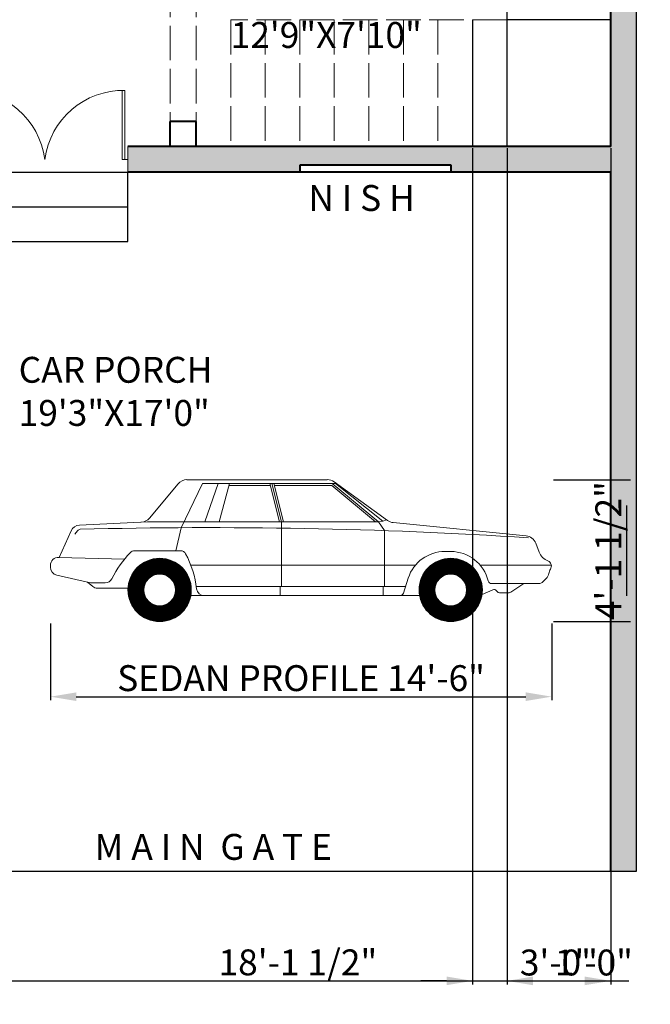
# Model space of a CAD drawing. Units: inches. Extents: x 1967493 to 1968177, y 907234 to 908105.
# Tile 3 of 5: x 1967854 to 1968074, y 907234 to 907576. Entities that reach past the tile are written whole.
import ezdxf

# ---------------------------------------------------------------- set-up
doc = ezdxf.new("R2010")
doc.units = ezdxf.units.IN
doc.linetypes.add('ACAD_ISO02W100', pattern=[15, 12, -3])
for name, color, linetype, lineweight in [('A-ANNO-DIMS', 2, 'Continuous', 18), ('A-ANNO-TEXT', 7, 'Continuous', 18), ('A-AREA-IDEN', 7, 'Continuous', 25), ('A-DOOR', 3, 'Continuous', 20), ('A-FLOR-STRS', 7, 'Continuous', 25), ('A-FLOR-STRS-HIDN', 7, 'ACAD_ISO02W100', 18), ('A-SITE-VEHL', 8, 'Continuous', 18), ('A-WALL', 7, 'Continuous', 40), ('A-WALL-OVHD', 7, 'ACAD_ISO02W100', 18), ('C-PROP', 7, 'Continuous', 25)]:
    doc.layers.add(name, color=color, linetype=linetype, lineweight=lineweight)
doc.layers.add('A-WALL-PATT', color=18, linetype='Continuous', lineweight=13, true_color=0x000000)
doc.styles.get("Standard").update_dxf_attribs({"font": 'arial.ttf'})
doc.dimstyles.new('ISO-25', dxfattribs={"dimtxt": 9, "dimasz": 9, "dimexe": 1.25, "dimexo": 0.625, "dimtad": 1, "dimdec": 1, "dimrnd": 9, "dimlunit": 3, "dimtxsty": 'Standard', "dimcen": 2.5, "dimadec": 0, "dimazin": 0, "dimtfac": 1, "dimtdec": 1, "dimtmove": 0, "dimatfit": 3, "dimfxl": 1, "dimarcsym": 0})

# ---------------------------------------------------------------- blocks, each defined once
blk = doc.blocks.new('Car - sedan  side')
for p, q in [((-128.57, 32.64), (-121.22, 48.02)), ((-77.81, 49.34), (-126.58, 49.34)), ((-74.7, 48.02), (-121.22, 48.02)), ((-120.32, 34.67), (-115.67, 48.02)), ((-115.4, 34.67), (-111.74, 48.02)), ((-94.41, 34.67), (-97.73, 48.02)), ((-93.72, 34.67), (-97.04, 48.02)), ((-93.03, 34.67), (-96.34, 48.02)), ((-60.02, 34.65), (-76.07, 48.02)), ((-56.87, 35.13), (-75.48, 48.59)), ((-58.54, 34.93), (-74.99, 48.02)), ((-139.53, 35.99), (-129.64, 47.91)), ((-97.55, 47.3), (-111.94, 47.3)), ((-76.26, 47.3), (-96.16, 47.3)), ((-61.08, 34.66), (-76.26, 47.3)), ((-140.23, 34.67), (-163.88, 33.56)), ((-62.28, 34.67), (-140.23, 34.67)), ((-93.72, 19.62), (-93.72, 34.67)), ((-62.28, 34.67), (-60.02, 34.65)), ((-60.02, 34.65), (-58.54, 34.93)), ((-57.97, 31.61), (-60.02, 34.65)), ((-57.21, 35.38), (-58.54, 34.93)), ((-54.93, 34.4), (-8.75, 29.8)), ((-170.93, 22.32), (-166.81, 31.56)), ((-164.57, 31.6), (-165.48, 30.35)), ((-130.39, 24.63), (-128.57, 32.64)), ((-57.97, 19.62), (-57.97, 31.61)), ((-128.78, 24.63), (-144.79, 24.63)), ((-36.97, 24.38), (-34.94, 24.38)), ((-4.21, 24.18), (-5.42, 27.27)), ((-148.26, 21.7), (-171.11, 22.33)), ((-174, 19.51), (-174, 18.91)), ((-47.2, 19.62), (-125.23, 19.62)), ((-93.72, 12.14), (-93.72, 19.62)), ((-57.97, 12.14), (-57.97, 19.62)), ((0, 19.62), (-24.7, 19.62)), ((-160.12, 13.48), (-171.81, 16.16)), ((-159.22, 12.14), (-161.08, 13.7)), ((-51.4, 9.89), (-49.69, 15.14)), ((-3.22, 13.59), (-1.77, 14.97)), ((-155.01, 13.48), (-160.12, 13.48)), ((-147.03, 11.6), (-157.73, 11.6)), ((-50.67, 12.14), (-123.32, 12.14)), ((-94.21, 9.03), (-94.21, 12.14)), ((-58.39, 9.03), (-58.39, 12.14)), ((-20.36, 11.06), (-24.06, 9.44)), ((-4.23, 13.19), (-20.72, 13.19)), ((-18.83, 10.42), (-19.11, 10.76)), ((-9.5, 13.19), (-14.1, 10.2)), ((-120.62, 9.03), (-125.23, 9.03)), ((-45.76, 9.03), (-120.62, 9.03)), ((-14.68, 10.03), (-18.01, 10.03))]:
    blk.add_line(p, q)
at = {"const_width": 5.49}
for points in [[(-127.8, 11, -1), (-144.3, 11, -1)], [(-26.69, 11, -1), (-43.19, 11, -1)]]:
    blk.add_lwpolyline(points, format="xyb", close=True, dxfattribs=at)
for centre, radius in [((-136.05, 11), 11), ((-34.94, 11), 11), ((-136.05, 11), 5.51), ((-34.94, 11), 5.51)]:
    blk.add_circle(centre, radius)
for centre, radius, start, end in [((-126.58, 45.38), 3.97, 90, 140.3029), ((-77.81, 45.38), 3.97, 54.135, 90), ((-142.58, 38.53), 3.97, 272.6827, 320.3029), ((-54.54, 38.35), 3.97, 234.135, 264.3123), ((-163.72, 30.18), 3.38, 92.6827, 155.9736), ((-163.62, 30.91), 1.17, 91.491, 143.9553), ((-118.51, -1702.12), 1734.79, 86.34698, 91.49105), ((-9.15, 25.82), 4, 21.3107, 84.3123), ((-118.09, -2.78), 38.85, 136.3964, 152.9097), ((-144.79, 22.64), 1.98, 90, 136.3964), ((-128.78, 22.64), 1.98, 28.1371, 90), ((-36.97, 11), 13.38, 90, 161.9732), ((-34.94, 11), 13.38, 13.5864, 90), ((0.9, 26.18), 5.49, 201.3107, 247.7048), ((-171.18, 19.51), 2.82, 88.4193, 180), ((-157.14, 7.48), 34.14, 6.5135, 28.1371), ((-1.92, 19.3), 1.94, 325.3744, 67.7048), ((-171.18, 18.91), 2.82, 180, 257.0905), ((2.46, 16.28), 3.37, 145.3744, 172.3839), ((-155.01, 16.1), 2.62, 270, 332.9097), ((-20.72, 14.43), 1.24, 193.5864, 270), ((-3.82, 17.12), 2.96, 313.7173, 352.3839), ((-157.73, 13.93), 2.32, 230.1291, 270), ((-120.62, 11.65), 2.62, 186.5135, 270), ((-19.93, 10.09), 1.06, 39.301, 113.7159), ((-18.01, 11.09), 1.06, 219.301, 270), ((-4.23, 14.65), 1.46, 270, 313.7173), ((-52.58, 10.27), 1.24, 270, 341.9732), ((-14.68, 11.09), 1.06, 270, 303.047)]:
    blk.add_arc(centre, radius, start, end)
blk = doc.blocks.new('*D44')
at = {"layer": 'A-ANNO-DIMS', "color": 0, "lineweight": -2, "transparency": 16777216}
for p, q in [((1967865.16, 907366.33), (1967865.16, 907339.59)), ((1968039.28, 907366.33), (1968039.28, 907339.59)), ((1967874.16, 907340.84), (1968030.28, 907340.84))]:
    blk.add_line(p, q, dxfattribs=at)
at = {"layer": 'A-ANNO-DIMS', "color": 0, "transparency": 16777216}
for points in [[(1967874.16, 907342.34), (1967874.16, 907339.34), (1967865.16, 907340.84)], [(1968030.28, 907342.34), (1968030.28, 907339.34), (1968039.28, 907340.84)]]:
    blk.add_solid(points, dxfattribs=at)
at = {"layer": 'Defpoints', "color": 0, "transparency": 16777216}
for p in [(1967865.16, 907366.96), (1968039.28, 907366.96), (1968039.28, 907340.84)]:
    blk.add_point(p, dxfattribs=at)
at = {"layer": 'A-ANNO-DIMS', "color": 0, "transparency": 16777216, "insert": (1967952.22, 907346.12), "char_height": 9, "attachment_point": 5}
blk.add_mtext('SEDAN PROFILE 14\'-6"', dxfattribs=at)
blk = doc.blocks.new('*D45')
at = {"layer": 'A-ANNO-DIMS', "color": 0, "lineweight": -2, "transparency": 16777216}
for p, q in [((1968039.9, 907416.3), (1968066.64, 907416.3)), ((1968065.39, 907375.96), (1968065.39, 907407.3)), ((1968039.9, 907366.96), (1968066.64, 907366.96))]:
    blk.add_line(p, q, dxfattribs=at)
at = {"layer": 'A-ANNO-DIMS', "color": 0, "transparency": 16777216}
for points in [[(1968063.89, 907407.3), (1968066.89, 907407.3), (1968065.39, 907416.3)], [(1968063.89, 907375.96), (1968066.89, 907375.96), (1968065.39, 907366.96)]]:
    blk.add_solid(points, dxfattribs=at)
at = {"layer": 'Defpoints', "color": 0, "transparency": 16777216}
for p in [(1968039.28, 907416.3), (1968065.39, 907416.3), (1968039.28, 907366.96)]:
    blk.add_point(p, dxfattribs=at)
at = {"layer": 'A-ANNO-DIMS', "color": 0, "transparency": 16777216, "insert": (1968060.12, 907391.63), "char_height": 9, "attachment_point": 5, "rotation": 90}
blk.add_mtext('4\'-1 1/2"', dxfattribs=at)
blk = doc.blocks.new('*D46')
at = {"layer": 'A-ANNO-DIMS', "color": 0, "lineweight": -2, "transparency": 16777216}
for p, q in [((1967842.47, 907279.54), (1967842.47, 907240.77)), ((1968059.78, 907279.54), (1968059.78, 907240.77)), ((1967851.47, 907242.02), (1968050.78, 907242.02))]:
    blk.add_line(p, q, dxfattribs=at)
at = {"layer": 'A-ANNO-DIMS', "color": 0, "transparency": 16777216}
for points in [[(1967851.47, 907243.52), (1967851.47, 907240.52), (1967842.47, 907242.02)], [(1968050.78, 907243.52), (1968050.78, 907240.52), (1968059.78, 907242.02)]]:
    blk.add_solid(points, dxfattribs=at)
at = {"layer": 'Defpoints', "color": 0, "transparency": 16777216}
for p in [(1967842.47, 907280.17), (1968059.78, 907280.17), (1968059.78, 907242.02)]:
    blk.add_point(p, dxfattribs=at)
at = {"layer": 'A-ANNO-DIMS', "color": 0, "transparency": 16777216, "insert": (1967951.12, 907247.29), "char_height": 9, "attachment_point": 5}
blk.add_mtext('18\'-1 1/2"', dxfattribs=at)
blk = doc.blocks.new('*D49')
at = {"layer": 'A-ANNO-DIMS', "color": 0, "lineweight": -2, "transparency": 16777216}
for p, q in [((1968023.78, 907531.54), (1968023.78, 907240.77)), ((1968059.78, 907531.54), (1968059.78, 907240.77)), ((1968032.78, 907242.02), (1968050.78, 907242.02))]:
    blk.add_line(p, q, dxfattribs=at)
at = {"layer": 'A-ANNO-DIMS', "color": 0, "transparency": 16777216}
for points in [[(1968032.78, 907243.52), (1968032.78, 907240.52), (1968023.78, 907242.02)], [(1968050.78, 907243.52), (1968050.78, 907240.52), (1968059.78, 907242.02)]]:
    blk.add_solid(points, dxfattribs=at)
at = {"layer": 'Defpoints', "color": 0, "transparency": 16777216}
for p in [(1968023.78, 907532.17), (1968059.78, 907532.17), (1968059.78, 907242.02)]:
    blk.add_point(p, dxfattribs=at)
at = {"layer": 'A-ANNO-DIMS', "color": 0, "transparency": 16777216, "insert": (1968041.78, 907247.24), "char_height": 9, "attachment_point": 5}
blk.add_mtext('3\'-0"', dxfattribs=at)
blk = doc.blocks.new('*D50')
at = {"layer": 'A-ANNO-DIMS', "color": 0, "lineweight": -2, "transparency": 16777216}
for p, q in [((1968011.78, 907531.54), (1968011.78, 907240.77)), ((1968023.78, 907531.54), (1968023.78, 907240.77)), ((1968002.78, 907242.02), (1967993.78, 907242.02)), ((1968011.78, 907242.02), (1968023.78, 907242.02)), ((1968032.78, 907242.02), (1968066.11, 907242.02))]:
    blk.add_line(p, q, dxfattribs=at)
at = {"layer": 'A-ANNO-DIMS', "color": 0, "transparency": 16777216}
for points in [[(1968002.78, 907243.52), (1968002.78, 907240.52), (1968011.78, 907242.02)], [(1968032.78, 907243.52), (1968032.78, 907240.52), (1968023.78, 907242.02)]]:
    blk.add_solid(points, dxfattribs=at)
at = {"layer": 'Defpoints', "color": 0, "transparency": 16777216}
for p in [(1968011.78, 907532.17), (1968023.78, 907532.17), (1968023.78, 907242.02)]:
    blk.add_point(p, dxfattribs=at)
at = {"layer": 'A-ANNO-DIMS', "color": 0, "transparency": 16777216, "insert": (1968053.94, 907247.24), "char_height": 9, "attachment_point": 5}
blk.add_mtext('1\'-0"', dxfattribs=at)

msp = doc.modelspace()

# ---------------------------------------------------------------- hatches: boundary and pattern name
at = {"layer": 'A-WALL-PATT'}
h = msp.add_hatch(color=256, dxfattribs=at)
h.dxf.hatch_style = 1
h.paths.add_polyline_path([(1967597.78, 907991.17), (1967717.78, 907991.17), (1967717.78, 907980.85), (1967726.78, 907980.85), (1967726.78, 907991.17), (1967885.78, 907991.17), (1967885.78, 907978.94), (1967894.78, 907978.94), (1967894.78, 907991.17), (1968059.78, 907991.17), (1968059.78, 907943.17), (1968039.39, 907943.17), (1968039.39, 907934.17), (1968059.78, 907934.17), (1968059.78, 907790.17), (1968052.82, 907790.17), (1968052.82, 907781.17), (1968059.78, 907781.17), (1968059.78, 907635.17), (1968052.82, 907635.17), (1968052.82, 907626.17), (1968059.78, 907626.17), (1968059.78, 907532.17), (1967892.06, 907532.17), (1967892.06, 907523.17), (1967951.97, 907523.17), (1967951.97, 907525.77), (1968004.23, 907525.77), (1968004.23, 907523.17), (1968059.78, 907523.17), (1968059.78, 907280.17), (1968068.78, 907280.17), (1968068.78, 908000.17), (1967588.78, 908000.17), (1967588.78, 907334.17), (1967828.78, 907334.17), (1967828.78, 907349.71), (1967819.78, 907349.71), (1967819.78, 907343.17), (1967597.78, 907343.17), (1967597.78, 907475.17), (1967774.78, 907475.17), (1967774.78, 907487.51), (1967765.78, 907487.51), (1967765.78, 907479.67), (1967597.78, 907479.67), (1967597.78, 907527.67), (1967604.66, 907527.67), (1967604.66, 907532.17), (1967597.78, 907532.17), (1967597.78, 907790.17), (1967597.78, 907934.17), (1967607.68, 907934.17), (1967607.68, 907943.17), (1967597.78, 907943.17)])
h.paths.add_polyline_path([(1967726.78, 907956.85), (1967717.78, 907956.85), (1967717.78, 907943.17), (1967726.78, 907943.17)], flags=17)
h.paths.add_polyline_path([(1967731.77, 907943.17), (1967651.01, 907943.17), (1967639.17, 907943.17), (1967639.17, 907934.17), (1967651.01, 907934.17), (1967731.77, 907934.17)], flags=17)
h.paths.add_polyline_path([(1967810.78, 907895.17), (1967774.78, 907895.17), (1967774.78, 907903.7), (1967765.78, 907903.7), (1967765.78, 907849.82), (1967765.78, 907834.76), (1967774.78, 907834.76), (1967774.78, 907849.82), (1967774.78, 907886.17), (1967810.78, 907886.17)], flags=17)
h.paths.add_polyline_path([(1967855.78, 907903.7), (1967846.78, 907903.7), (1967846.78, 907895.17), (1967845.59, 907895.17), (1967845.59, 907886.17), (1967846.78, 907886.17), (1967846.78, 907849.82), (1967846.78, 907834.76), (1967855.78, 907834.76), (1967855.78, 907849.82)], flags=17)
h.paths.add_polyline_path([(1968003.67, 907943.17), (1967999.78, 907943.17), (1967999.78, 907946.67), (1967990.78, 907946.67), (1967990.78, 907943.17), (1967881.11, 907943.17), (1967881.11, 907934.17), (1968003.67, 907934.17)], flags=17)
h.paths.add_polyline_path([(1967999.78, 907991.17), (1967990.78, 907991.17), (1967990.78, 907969.75, -0.052013), (1967995.28, 907969.73), (1967999.78, 907969.73)], flags=17)
h.paths.add_polyline_path([(1967777.59, 907790.17), (1967774.78, 907790.17), (1967774.78, 907796.26), (1967765.78, 907796.26), (1967765.78, 907790.17), (1967648.78, 907790.17), (1967648.78, 907769.17), (1967597.78, 907769.17), (1967597.78, 907760.17), (1967648.78, 907760.17), (1967648.78, 907749.33), (1967657.78, 907749.33), (1967657.78, 907781.17), (1967765.78, 907781.17), (1967765.78, 907721), (1967774.78, 907721), (1967774.78, 907781.17), (1967777.59, 907781.17)], flags=17)
h.paths.add_polyline_path([(1968016.82, 907790.17), (1967855.78, 907790.17), (1967855.78, 907796.26), (1967846.78, 907796.26), (1967846.78, 907790.17), (1967843.5, 907790.17), (1967843.5, 907781.17), (1967855.78, 907781.17), (1968002.78, 907781.17), (1968002.78, 907767.09), (1968011.78, 907767.09), (1968011.78, 907781.17), (1968016.82, 907781.17)], flags=17)
h.paths.add_polyline_path([(1968011.78, 907731.09), (1968002.78, 907731.09), (1968002.78, 907698.5), (1968011.78, 907698.5)], flags=17)
h.paths.add_polyline_path([(1968011.78, 907662.5), (1968002.78, 907662.5), (1968002.78, 907635.17), (1967892.06, 907635.17), (1967892.06, 907626.17), (1968016.82, 907626.17), (1968016.82, 907635.17), (1968011.78, 907635.17)], flags=17)
h.paths.add_polyline_path([(1967774.78, 907679.04), (1967765.78, 907679.04), (1967765.78, 907673.17), (1967657.78, 907673.17), (1967657.78, 907679.08), (1967648.78, 907679.08), (1967648.78, 907673.17), (1967639.33, 907673.17), (1967639.33, 907664.17), (1967765.78, 907664.17), (1967765.78, 907577.1), (1967768.96, 907577.1, -0.009361), (1967770.28, 907577.1), (1967774.78, 907577.1), (1967774.78, 907626.17), (1967779.99, 907626.17), (1967779.99, 907635.17), (1967774.78, 907635.17)], flags=17)
h.paths.add_polyline_path([(1967603.33, 907673.17), (1967597.78, 907673.17), (1967597.78, 907664.17), (1967603.33, 907664.17)], flags=17)
h.paths.add_polyline_path([(1967774.78, 907540.27), (1967765.78, 907540.27), (1967765.78, 907532.17), (1967644.82, 907532.17), (1967644.82, 907527.67), (1967765.78, 907527.67), (1967765.78, 907522.83), (1967774.78, 907522.83)], flags=17)
h.paths.add_polyline_path([(1967828.78, 907475.17), (1967828.78, 907479.67), (1967828.78, 907523.17), (1967834.39, 907523.17), (1967834.39, 907532.17), (1967828.78, 907532.17), (1967813.83, 907532.17), (1967813.83, 907527.67), (1967819.78, 907527.67), (1967819.78, 907479.67), (1967819.78, 907475.17), (1967819.78, 907388.61), (1967828.78, 907388.61)], flags=17)

# ---------------------------------------------------------------- linework, layer by layer
at = {"layer": 'A-DOOR'}
for p, q in [((1967891.06, 907551.67), (1967890.06, 907551.67)), ((1967890.06, 907551.67), (1967890.06, 907527.67)), ((1967891.06, 907527.67), (1967891.06, 907551.67)), ((1967890.06, 907527.67), (1967891.56, 907527.67)), ((1967892.06, 907527.67), (1967891.06, 907527.67))]:
    msp.add_line(p, q, dxfattribs=at)
for centre, start, end in [((1967835.89, 907524.1), 7.4241, 91.0393), ((1967890.56, 907524.1), 88.9607, 172.5759)]:
    msp.add_arc(centre, 27.57, start, end, dxfattribs=at)
at = {"layer": 'A-FLOR-STRS'}
for p, q in [((1968023.78, 907532.17), (1968023.78, 907626.17)), ((1968011.78, 907576.17), (1968011.78, 907532.17)), ((1968059.78, 907576.17), (1968023.78, 907576.17)), ((1967834.39, 907523.17), (1967892.06, 907523.17)), ((1967892.06, 907499.17), (1967892.06, 907523.17)), ((1967834.39, 907511.17), (1967892.06, 907511.17)), ((1967834.39, 907499.17), (1967892.06, 907499.17))]:
    msp.add_line(p, q, dxfattribs=at)
at = {"layer": 'A-FLOR-STRS-HIDN'}
for p, q in [((1968023.78, 907576.17), (1967927.78, 907576.17)), ((1967927.78, 907576.17), (1967927.78, 907532.17)), ((1967939.78, 907576.17), (1967939.78, 907532.17)), ((1967951.78, 907576.17), (1967951.78, 907532.17)), ((1967963.78, 907576.17), (1967963.78, 907532.17)), ((1967975.78, 907576.17), (1967975.78, 907532.17)), ((1967987.78, 907576.17), (1967987.78, 907532.17)), ((1967999.78, 907576.17), (1967999.78, 907532.17))]:
    msp.add_line(p, q, dxfattribs=at)
at = {"layer": 'A-WALL'}
for p, q in [((1968059.78, 907532.17), (1968059.78, 907626.17)), ((1967906.78, 907532.17), (1967906.78, 907540.81)), ((1967915.78, 907540.81), (1967906.78, 907540.81)), ((1967915.78, 907532.17), (1967915.78, 907540.81)), ((1968059.78, 907532.17), (1967892.06, 907532.17)), ((1967951.97, 907523.17), (1967951.97, 907525.77)), ((1967951.97, 907525.77), (1968004.23, 907525.77)), ((1968004.23, 907525.77), (1968004.23, 907523.17)), ((1968059.78, 907523.17), (1967892.06, 907523.17)), ((1967951.97, 907523.17), (1967951.97, 907523.17)), ((1968059.78, 907280.17), (1968059.78, 907523.17))]:
    msp.add_line(p, q, dxfattribs=at)
at = {"layer": 'A-WALL-OVHD'}
for p, q in [((1967906.78, 907619.12), (1967906.78, 907540.81)), ((1967915.78, 907619.12), (1967915.78, 907540.81)), ((1967892.06, 907532.17), (1967892.06, 907523.17))]:
    msp.add_line(p, q, dxfattribs=at)
at = {"layer": 'C-PROP'}
for p, q in [((1968068.78, 907280.17), (1968068.78, 908000.17)), ((1967588.78, 907280.17), (1968068.78, 907280.17))]:
    msp.add_line(p, q, dxfattribs=at)

# ---------------------------------------------------------------- block references
at = {"layer": 'A-SITE-VEHL'}
msp.add_blockref('Car - sedan  side', (1968039.16, 907366.96), dxfattribs=at)

# ---------------------------------------------------------------- texts
at = {"layer": 'A-ANNO-TEXT', "char_height": 9, "attachment_point": 1}
for s, width, insert in [('N I S H', 47.4714, (1967954.77, 907518.74)), ('M A I N  G A T E', 155.8771, (1967880.54, 907293.11))]:
    msp.add_mtext_dynamic_manual_height_columns(s, width=width, gutter_width=12.5, heights=[0], dxfattribs=dict(at, insert=insert))
at = {"layer": 'A-AREA-IDEN', "char_height": 9, "attachment_point": 1}
for s, width, insert in [('STAIR BOX\\P12\'9"X7\'10"', 82.0284, (1967927.78, 907590.43)), ('CAR PORCH\\P19\'3"X17\'0"', 75.7536, (1967854.13, 907459))]:
    msp.add_mtext_dynamic_manual_height_columns(s, width=width, gutter_width=12.5, heights=[0], dxfattribs=dict(at, insert=insert))

# ---------------------------------------------------------------- dimensions: what is measured, and where the dimension line sits
at = {"layer": 'A-ANNO-DIMS'}
for base, p1, p2, picture, middle in [((1968023.78, 907242.02), (1968011.78, 907532.17), (1968023.78, 907532.17), '*D50', (1968053.94, 907247.24)), ((1968059.78, 907242.02), (1968023.78, 907532.17), (1968059.78, 907532.17), '*D49', (1968041.78, 907247.24)), ((1968059.78, 907242.02), (1967842.47, 907280.17), (1968059.78, 907280.17), '*D46', (1967951.12, 907247.29))]:
    dim = msp.add_linear_dim(base=base, p1=p1, p2=p2, dimstyle='ISO-25', override={"dimdec": 1, "dimlfac": 1, "dimrnd": 0, "dimzin": 1, "dimdsep": 46, "dimlunit": 4, "dimfrac": 2}, dxfattribs=at)
    dim.commit()
    dim.dimension.update_dxf_attribs({"geometry": picture, "text_midpoint": middle})
dim = msp.add_linear_dim(base=(1968065.39, 907416.3), p1=(1968039.28, 907366.96), p2=(1968039.28, 907416.3), angle=90, dimstyle='ISO-25', override={"dimdec": 1, "dimlfac": 1, "dimrnd": 0, "dimzin": 1, "dimdsep": 46, "dimlunit": 4, "dimfrac": 2}, dxfattribs=at)
dim.commit()
dim.dimension.update_dxf_attribs({"geometry": '*D45', "text_midpoint": (1968060.12, 907391.63)})
dim = msp.add_linear_dim(base=(1968039.28, 907340.84), p1=(1967865.16, 907366.96), p2=(1968039.28, 907366.96), text='SEDAN PROFILE <>', dimstyle='ISO-25', override={"dimdec": 1, "dimlfac": 1, "dimrnd": 0, "dimzin": 1, "dimdsep": 46, "dimlunit": 4, "dimfrac": 2}, dxfattribs=at)
dim.commit()
dim.dimension.update_dxf_attribs({"geometry": '*D44', "text_midpoint": (1967952.22, 907346.12)})

doc.saveas('drawing.dxf')
